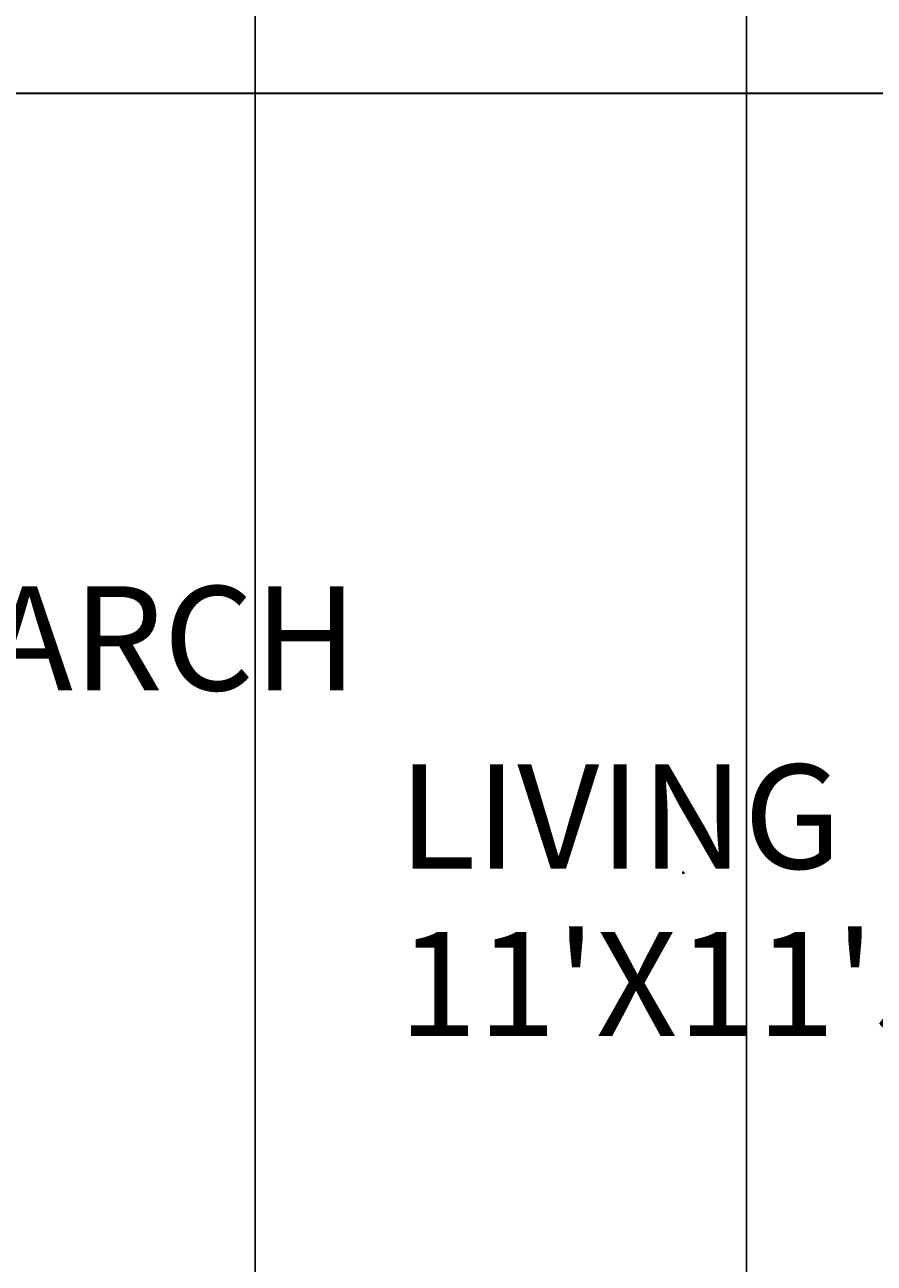
# Model space of a CAD drawing. Units: feet. Extents: x 1654 to 2985, y 1348 to 2230.
# Tile 46 of 53: x 2655 to 2723, y 1792 to 1892. Entities that reach past the tile are written whole.
import ezdxf

# ---------------------------------------------------------------- set-up
doc = ezdxf.new("R2010")
doc.units = ezdxf.units.FT
for name, color, linetype, lineweight in [('A-ANNO-DIMS', 2, 'Continuous', 18), ('A-ANNO-TEXT', 7, 'Continuous', 18), ('A-AREA-IDEN', 7, 'Continuous', 18), ('A-WALL', 7, 'Continuous', 35)]:
    doc.layers.add(name, color=color, linetype=linetype, lineweight=lineweight)
doc.styles.get("Standard").update_dxf_attribs({"font": 'arial.ttf'})
doc.dimstyles.get("Standard").update_dxf_attribs({"dimtxt": 0.18, "dimasz": 0.18, "dimexe": 0.18, "dimexo": 0.0625, "dimgap": 0.09, "dimtad": 0, "dimtih": 1, "dimtoh": 1, "dimdec": 4, "dimzin": 0, "dimdsep": 46, "dimtxsty": 'Standard', "dimcen": 0.09, "dimadec": 0, "dimazin": 0, "dimtfac": 1, "dimtdec": 4, "dimtofl": 0, "dimtmove": 0, "dimatfit": 3, "dimfxl": 1, "dimtolj": 1, "dimtzin": 0, "dimarcsym": 0})

# ---------------------------------------------------------------- blocks, each defined once
blk = doc.blocks.new('*D82')
at = {"layer": 'A-ANNO-DIMS', "color": 0, "lineweight": -2, "transparency": 16777216}
for p, q in [((2652.706, 2039.192), (2652.706, 1490.625)), ((2784.706, 2039.192), (2784.706, 1490.625)), ((2652.886, 1490.805), (2718.426, 1490.805)), ((2784.526, 1490.805), (2718.985, 1490.805))]:
    blk.add_line(p, q, dxfattribs=at)
at = {"layer": 'A-ANNO-DIMS', "color": 0, "transparency": 16777216}
for points in [[(2652.886, 1490.835), (2652.886, 1490.775), (2652.706, 1490.805)], [(2784.526, 1490.835), (2784.526, 1490.775), (2784.706, 1490.805)]]:
    blk.add_solid(points, dxfattribs=at)
at = {"layer": 'Defpoints', "color": 0, "transparency": 16777216}
for p in [(2652.706, 2039.255), (2784.706, 2039.255), (2784.706, 1490.805)]:
    blk.add_point(p, dxfattribs=at)
at = {"layer": 'A-ANNO-DIMS', "color": 0, "transparency": 16777216, "insert": (2718.706, 1490.805), "char_height": 0.18, "attachment_point": 5}
blk.add_mtext('\\A1;132', dxfattribs=at)
blk = doc.blocks.new('*D84')
at = {"layer": 'A-ANNO-DIMS', "color": 0, "lineweight": -2, "transparency": 16777216}
for p, q in [((2625.235, 1565.317), (2625.235, 2149.885)), ((2625.415, 2149.705), (2649.013, 2149.705)), ((2673.055, 2149.705), (2649.458, 2149.705)), ((2673.235, 1565.317), (2673.235, 2149.885))]:
    blk.add_line(p, q, dxfattribs=at)
at = {"layer": 'A-ANNO-DIMS', "color": 0, "transparency": 16777216}
for points in [[(2625.415, 2149.735), (2625.415, 2149.675), (2625.235, 2149.705)], [(2673.055, 2149.735), (2673.055, 2149.675), (2673.235, 2149.705)]]:
    blk.add_solid(points, dxfattribs=at)
at = {"layer": 'Defpoints', "color": 0, "transparency": 16777216}
for p in [(2673.235, 2149.705), (2625.235, 1565.255), (2673.235, 1565.255)]:
    blk.add_point(p, dxfattribs=at)
at = {"layer": 'A-ANNO-DIMS', "color": 0, "transparency": 16777216, "insert": (2649.235, 2149.705), "char_height": 0.18, "attachment_point": 5}
blk.add_mtext('\\A1;48', dxfattribs=at)
blk = doc.blocks.new('*D85')
at = {"layer": 'A-ANNO-DIMS', "color": 0, "lineweight": -2, "transparency": 16777216}
for p, q in [((2673.235, 1565.317), (2673.235, 2149.885)), ((2673.415, 2149.705), (2692.577, 2149.705)), ((2712.526, 2149.705), (2693.364, 2149.705)), ((2712.706, 1565.317), (2712.706, 2149.885))]:
    blk.add_line(p, q, dxfattribs=at)
at = {"layer": 'A-ANNO-DIMS', "color": 0, "transparency": 16777216}
for points in [[(2673.415, 2149.735), (2673.415, 2149.675), (2673.235, 2149.705)], [(2712.526, 2149.735), (2712.526, 2149.675), (2712.706, 2149.705)]]:
    blk.add_solid(points, dxfattribs=at)
at = {"layer": 'Defpoints', "color": 0, "transparency": 16777216}
for p in [(2712.706, 2149.705), (2673.235, 1565.255), (2712.706, 1565.255)]:
    blk.add_point(p, dxfattribs=at)
at = {"layer": 'A-ANNO-DIMS', "color": 0, "transparency": 16777216, "insert": (2692.971, 2149.705), "char_height": 0.18, "attachment_point": 5}
blk.add_mtext('\\A1;39.47', dxfattribs=at)
blk = doc.blocks.new('*D109')
at = {"layer": 'A-ANNO-DIMS', "color": 0, "lineweight": -2, "transparency": 16777216}
for p, q in [((2707.634, 1823.491), (2707.634, 1823.671)), ((2707.544, 1823.581), (2707.724, 1823.581)), ((2825.812, 1823.581), (2781.675, 1823.581))]:
    blk.add_line(p, q, dxfattribs=at)
at = {"layer": 'A-ANNO-DIMS', "color": 0, "transparency": 16777216}
blk.add_solid([(2781.675, 1823.611), (2781.675, 1823.551), (2781.495, 1823.581)], dxfattribs=at)
at = {"layer": 'Defpoints', "color": 0, "transparency": 16777216}
for p in [(2707.634, 1823.581), (2781.495, 1823.581)]:
    blk.add_point(p, dxfattribs=at)
at = {"layer": 'A-ANNO-DIMS', "color": 0, "transparency": 16777216, "insert": (2826.486, 1823.581), "char_height": 0.18, "attachment_point": 5}
blk.add_mtext('\\A1;2X R73.86', dxfattribs=at)

msp = doc.modelspace()

# ---------------------------------------------------------------- linework, layer by layer
at = {"layer": 'A-WALL'}
msp.add_line((2784.7058, 1886.2549), (2652.7058, 1886.2549), dxfattribs=at)

# ---------------------------------------------------------------- texts
at = {"layer": 'A-ANNO-TEXT'}
msp.add_text('3\'6" ARCH', height=8.38114, dxfattribs=at).set_placement((2627.7728, 1838.2451))
at = {"layer": 'A-AREA-IDEN'}
for s, p in [('LIVING', (2684.7392, 1823.9066)), ('11\'X11\'3"', (2684.7392, 1810.4431))]:
    msp.add_text(s, height=8.38114, dxfattribs=at).set_placement(p)

# ---------------------------------------------------------------- dimensions: what is measured, and where the dimension line sits
at = {"layer": 'A-ANNO-DIMS'}
for base, p1, p2, override, picture, middle in [((2673.2353, 2149.7049), (2625.2353, 1565.2549), (2673.2353, 1565.2549), {"dimdec": 0, "dimlfac": 1, "dimrnd": 0, "dimzin": 0, "dimdsep": 46, "dimlunit": 2}, '*D84', (2649.2353, 2149.7049)), ((2712.7058, 2149.7049), (2673.2353, 1565.2549), (2712.7058, 1565.2549), {"dimdec": 2, "dimlfac": 1, "dimrnd": 0, "dimzin": 0, "dimdsep": 46, "dimlunit": 2}, '*D85', (2692.9706, 2149.7049)), ((2784.7058, 1490.8049), (2652.7058, 2039.2549), (2784.7058, 2039.2549), {"dimdec": 0, "dimlfac": 1, "dimrnd": 0, "dimzin": 0, "dimdsep": 46, "dimlunit": 2}, '*D82', (2718.7058, 1490.8049))]:
    dim = msp.add_linear_dim(base=base, p1=p1, p2=p2, dimstyle='Standard', override=override, dxfattribs=at)
    dim.commit()
    dim.dimension.update_dxf_attribs({"geometry": picture, "text_midpoint": middle})
dim = msp.add_radius_dim(center=(2707.634, 1823.581), mpoint=(2781.495, 1823.581), text='2X <>', dimstyle='Standard', override={"dimdec": 2, "dimlfac": 1, "dimrnd": 0, "dimzin": 0, "dimdsep": 46, "dimlunit": 2}, dxfattribs=at)
dim.commit()
dim.dimension.update_dxf_attribs({"geometry": '*D109', "text_midpoint": (2825.8115, 1823.581), "dimtype": 164})

doc.saveas('drawing.dxf')
